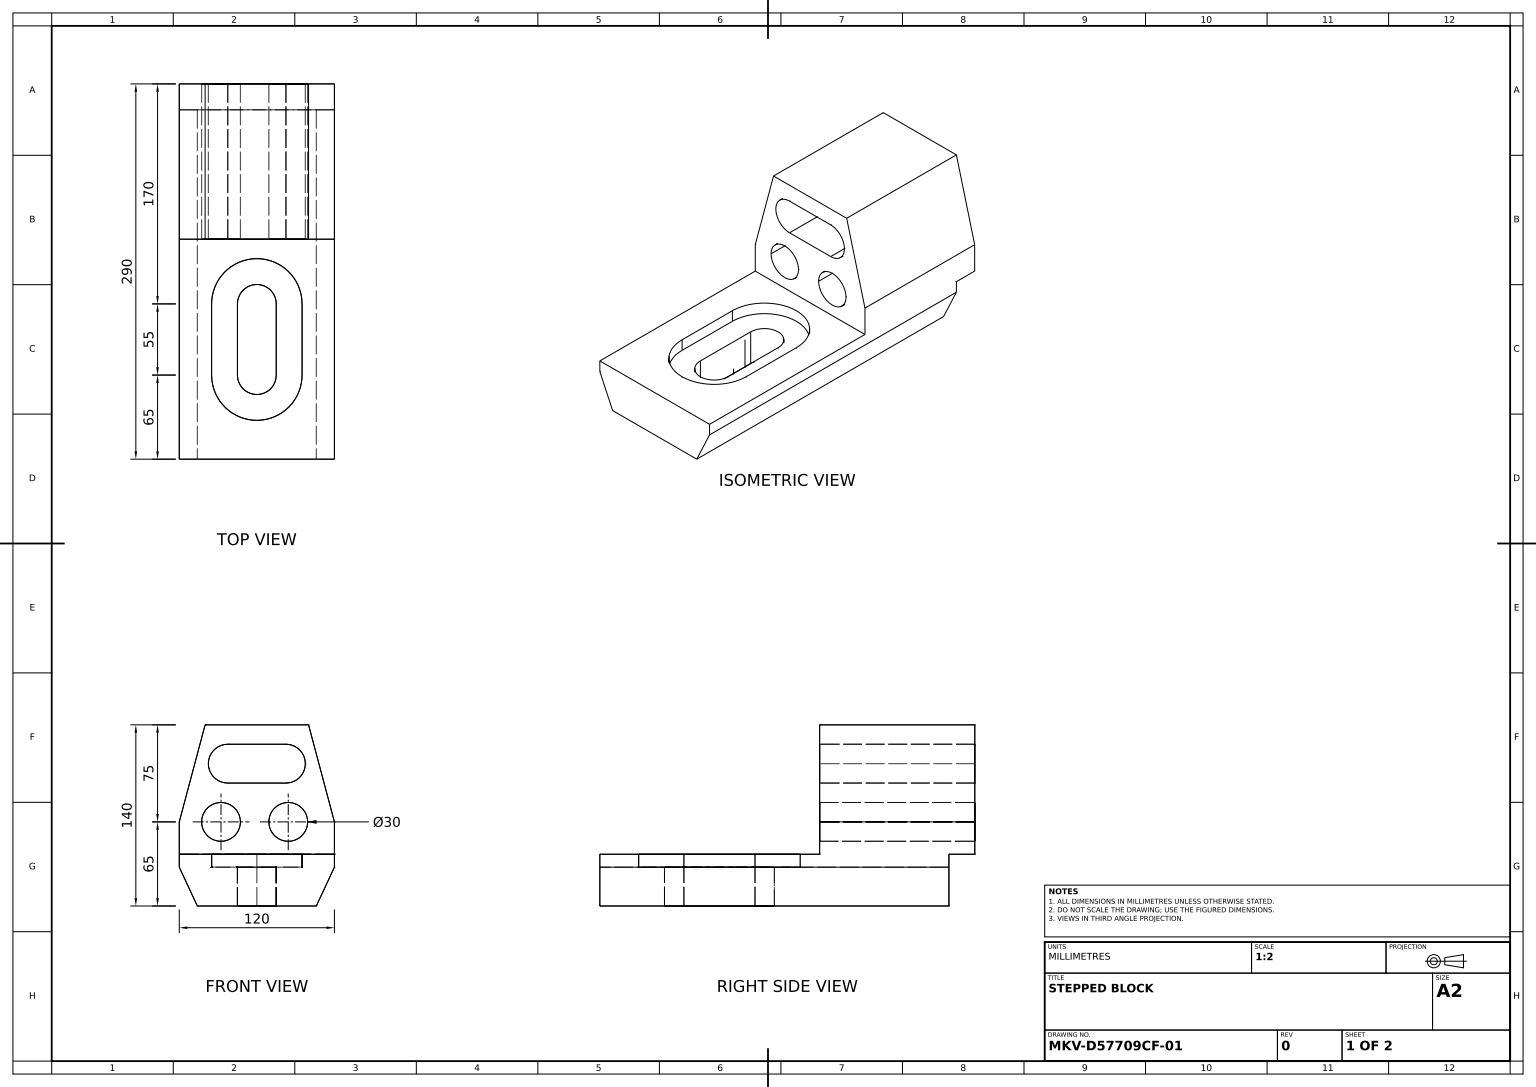
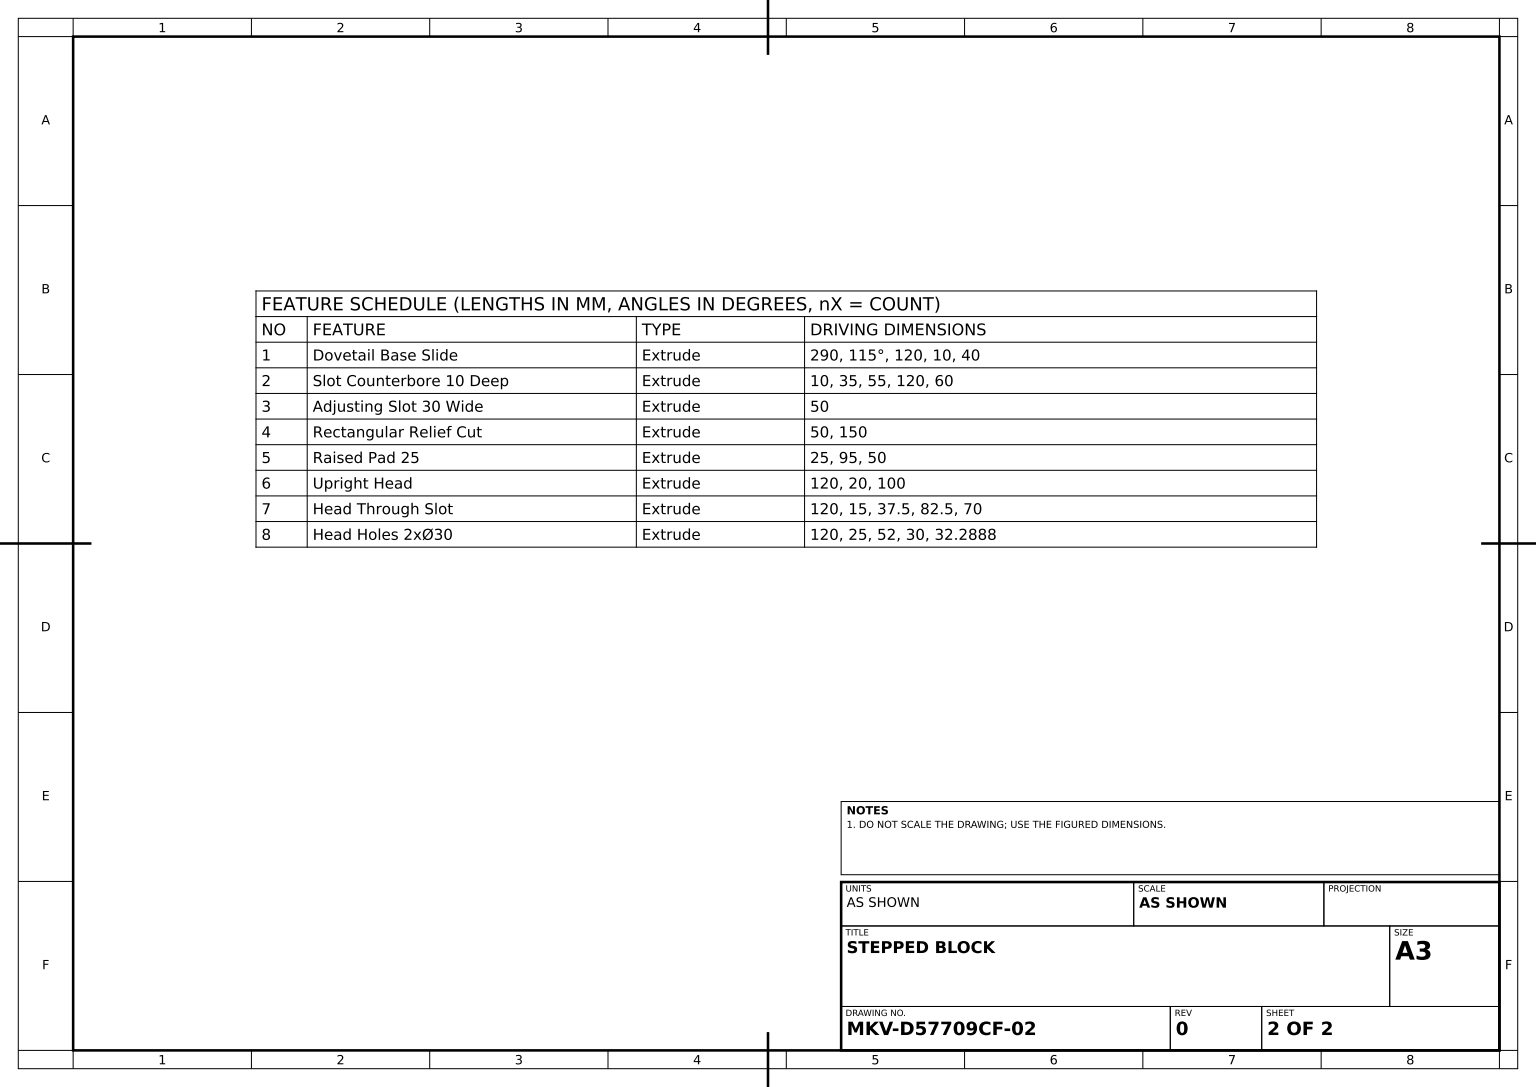
SolidWorks part; units mm, degrees
material "Plain Carbon Steel"
ref_plane "Front Plane" through (0, 0, 0) normal (0, 0, 1) x (1, 0, 0)
ref_plane "Top Plane" through (0, 0, 0) normal (0, 1, 0) x (1, 0, 0)
ref_plane "Right Plane" through (0, 0, 0) normal (1, 0, 0) x (0, 0, -1)
sketch "Dovetail Base Profile Sketch" plane through (0, 0, 0) normal (0, 0, 1) x (1, 0, 0)
  line L0 (0, 0) -> (92.0215, 0)
  line L1 (92.0215, 0) -> (106.0108, 30)
  line L2 (0, 0) -> (-13.9892, 30)
  line L3 (0, 0) -> (-13.9892, 30)
  line L5 (-13.9892, 30) -> (-13.9892, 40)
  line L6 (-13.9892, 40) -> (106.0108, 40)
  line L7 (106.0108, 40) -> (106.0108, 30)
  dimension "D1" = 115
  dimension "D2" = 115
  dimension "D3" = 40
  dimension "D4" = 120
  dimension "D5" = 10
  dimension "D6" = 120
extrude "Dovetail Base Slide" add sketch "Dovetail Base Profile Sketch" against normal blind 290 contours L7 L6 L5 L2 L0 L1
sketch "Slot Counterbore Sketch" plane through (0, 40, 0) normal (0, 1, 0) x (1, 0, 0)
  line L1 (106.0108, 290) -> (106.0108, 0) construction
  line L3 (11.0108, 120) -> (11.0108, 65)
  line L4 (81.0108, 120) -> (81.0108, 65)
  line L5 (-13.9892, 0) -> (106.0108, 0) construction
  arc A1 (81.0108, 120) -> (11.0108, 120) centre (46.0108, 120) ccw
  arc A2 (11.0108, 65) -> (81.0108, 65) centre (46.0108, 65) ccw
  dimension "D1" = 35
  dimension "D2" = 70
  dimension "D3" = 70
  dimension "D4" = 55
  dimension "D5" = 120
  dimension "D6" = 60
extrude "Slot Counterbore 10 Deep" cut sketch "Slot Counterbore Sketch" against normal blind 10
sketch "Adjusting Slot Sketch" plane through (0, 30, 0) normal (0, 1, 0) x (1, 0, 0)
  line L0 (31.0108, 120) -> (31.0108, 65)
  line L1 (61.0108, 120) -> (61.0108, 65)
  arc A0 (61.0108, 120) -> (31.0108, 120) centre (46.0108, 120) ccw
  arc A1 (31.0108, 65) -> (61.0108, 65) centre (46.0108, 65) ccw
  dimension "D1" = 30
  dimension "D2" = 30
extrude "Adjusting Slot 30 Wide" cut sketch "Adjusting Slot Sketch" against normal blind 50
sketch "Relief Cut Sketch" plane through (0, 40, 0) normal (0, 1, 0) x (1, 0, 0)
  line L1 (-13.9892, 290) -> (-13.9892, 0) construction
  line L4 (106.0108, 290) -> (106.0108, 0) construction
  line L6 (106.0108, 270) -> (-13.9892, 270)
  line L7 (-13.9892, 270) -> (-13.9892, 290)
  line L8 (-13.9892, 290) -> (106.0108, 290)
  line L9 (106.0108, 290) -> (106.0108, 270)
  dimension "D1" = 150
extrude "Rectangular Relief Cut" cut sketch "Relief Cut Sketch" against normal blind 50
sketch "Raised Pad Sketch" plane through (0, 40, 0) normal (0, 1, 0) x (1, 0, 0)
  line L0 (106.0108, 170) -> (106.0108, 290)
  line L1 (106.0108, 290) -> (-13.9892, 290)
  line L2 (11.0108, 120) -> (11.0108, 65) construction
  line L3 (-13.9892, 270) -> (-13.9892, 0) construction
  line L4 (-13.9892, 170) -> (106.0108, 170)
  line L5 (-13.9892, 290) -> (-13.9892, 170)
  dimension "D1" = 95
  dimension "D2" = 50
extrude "Raised Pad 25" add sketch "Raised Pad Sketch" along normal blind 25
sketch "Upright Head Profile Sketch" plane through (0, 0, -170) normal (0, 0, 1) x (1, 0, 0)
  line L0 (106.0108, 65) -> (106.0108, 40) construction
  line L1 (-13.9892, 40) -> (106.0108, 40) construction
  line L2 (46.0108, 140) -> (6.0108, 140)
  line L3 (6.0108, 140) -> (-13.9892, 65)
  line L4 (-13.9892, 65) -> (106.0108, 65)
  line L5 (46.0108, 140) -> (86.0108, 140)
  line L6 (86.0108, 140) -> (106.0108, 65)
  dimension "D1" = 20
  dimension "D2" = 100
extrude "Upright Head" add sketch "Upright Head Profile Sketch" against normal blind 120
sketch "Head Slot Sketch" plane through (0, 0, -170) normal (0, 0, 1) x (1, 0, 0)
  line L0 (106.0108, 65) -> (106.0108, 40) construction
  line L1 (-13.9892, 40) -> (106.0108, 40) construction
  line L4 (23.5108, 125) -> (68.5108, 125)
  line L5 (23.5108, 95) -> (68.5108, 95)
  arc A0 (23.5108, 125) -> (23.5108, 95) centre (23.5108, 110) ccw
  arc A1 (68.5108, 95) -> (68.5108, 125) centre (68.5108, 110) ccw
  dimension "D1" = 15
  dimension "D2" = 37.5
  dimension "D3" = 82.5
  dimension "D4" = 70
extrude "Head Through Slot" cut sketch "Head Slot Sketch" against normal blind 120
sketch "Head Holes Sketch" plane through (0, 0, -170) normal (0, 0, 1) x (1, 0, 0)
  line L0 (-13.9892, 40) -> (106.0108, 40) construction
  circle A0 centre (18.2996, 65) radius 15
  circle A1 centre (70.2996, 65) radius 15
  dimension "D1" = 30
  dimension "D2" = 30
  dimension "D6" = 30
  dimension "D3" = 25
  dimension "D4" = 25
  dimension "D5" = 52
  dimension "D7" = 32.2888
extrude "Head Holes 2xØ30" cut sketch "Head Holes Sketch" against normal blind 120
